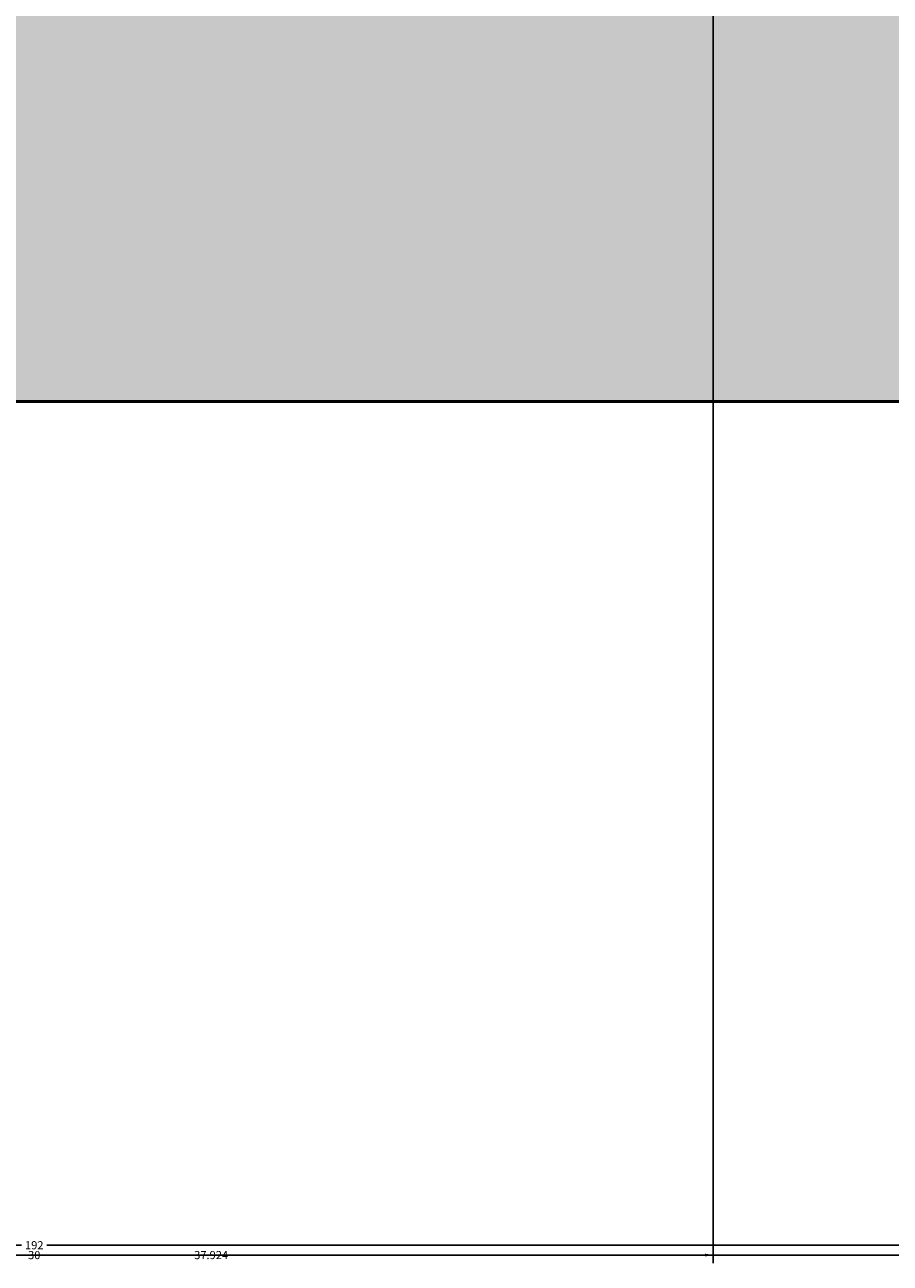
# Model space of a CAD drawing. Units: inches. Extents: x 2231 to 2461, y 2045 to 2455.
# Tile 14 of 95: x 2346 to 2365, y 2045 to 2072. Entities that reach past the tile are written whole.
import ezdxf

# ---------------------------------------------------------------- set-up
doc = ezdxf.new("R2010")
doc.units = ezdxf.units.IN
doc.layers.add('A-ANNO-DIMS', color=2, linetype='Continuous', lineweight=18)
doc.layers.add('A-WALL', color=7, linetype='Continuous', lineweight=50)
doc.layers.add('A-WALL-PATT', color=18, linetype='Continuous', lineweight=13, true_color=0x000000)
doc.styles.get("Standard").update_dxf_attribs({"font": 'arial.ttf'})
doc.dimstyles.get("Standard").update_dxf_attribs({"dimtxt": 0.18, "dimasz": 0.18, "dimexe": 0.18, "dimexo": 0.0625, "dimgap": 0.09, "dimtad": 0, "dimtih": 1, "dimtoh": 1, "dimdec": 4, "dimzin": 0, "dimdsep": 46, "dimtxsty": 'Standard', "dimcen": 0.09, "dimadec": 0, "dimazin": 0, "dimtfac": 1, "dimtdec": 4, "dimtofl": 0, "dimtmove": 0, "dimatfit": 3, "dimfxl": 1, "dimtolj": 1, "dimtzin": 0, "dimarcsym": 0})

# ---------------------------------------------------------------- blocks, each defined once
blk = doc.blocks.new('*D33')
at = {"layer": 'A-ANNO-DIMS', "color": 0, "lineweight": -2, "transparency": 16777216}
for p, q in [((2249.794, 2063.77), (2249.794, 2045.02)), ((2441.794, 2063.77), (2441.794, 2045.02)), ((2249.974, 2045.2), (2345.514, 2045.2)), ((2441.614, 2045.2), (2346.073, 2045.2))]:
    blk.add_line(p, q, dxfattribs=at)
at = {"layer": 'A-ANNO-DIMS', "color": 0, "transparency": 16777216}
for points in [[(2249.974, 2045.23), (2249.974, 2045.17), (2249.794, 2045.2)], [(2441.614, 2045.23), (2441.614, 2045.17), (2441.794, 2045.2)]]:
    blk.add_solid(points, dxfattribs=at)
at = {"layer": 'Defpoints', "color": 0, "transparency": 16777216}
for p in [(2249.794, 2063.833), (2441.794, 2063.833), (2249.794, 2045.2)]:
    blk.add_point(p, dxfattribs=at)
at = {"layer": 'A-ANNO-DIMS', "color": 0, "transparency": 16777216, "insert": (2345.794, 2045.2), "char_height": 0.18, "attachment_point": 5}
blk.add_mtext('\\A1;192', dxfattribs=at)
blk = doc.blocks.new('*D46')
at = {"layer": 'A-ANNO-DIMS', "color": 0, "lineweight": -2, "transparency": 16777216}
for p, q in [((2330.74, 2063.77), (2330.74, 2044.803)), ((2368.664, 2063.77), (2368.664, 2044.803)), ((2330.92, 2044.983), (2349.239, 2044.983)), ((2368.484, 2044.983), (2350.165, 2044.983))]:
    blk.add_line(p, q, dxfattribs=at)
at = {"layer": 'A-ANNO-DIMS', "color": 0, "transparency": 16777216}
for points in [[(2330.92, 2045.013), (2330.92, 2044.953), (2330.74, 2044.983)], [(2368.484, 2045.013), (2368.484, 2044.953), (2368.664, 2044.983)]]:
    blk.add_solid(points, dxfattribs=at)
at = {"layer": 'Defpoints', "color": 0, "transparency": 16777216}
for p in [(2330.74, 2063.833), (2368.664, 2063.833), (2368.664, 2044.983)]:
    blk.add_point(p, dxfattribs=at)
at = {"layer": 'A-ANNO-DIMS', "color": 0, "transparency": 16777216, "insert": (2349.702, 2044.983), "char_height": 0.18, "attachment_point": 5}
blk.add_mtext('\\A1;37.924', dxfattribs=at)
blk = doc.blocks.new('*D52')
at = {"layer": 'A-ANNO-DIMS', "color": 0, "lineweight": -2, "transparency": 16777216}
for p, q in [((2330.794, 2306.77), (2330.794, 2044.803)), ((2360.794, 2306.77), (2360.794, 2044.803)), ((2330.974, 2044.983), (2345.575, 2044.983)), ((2360.614, 2044.983), (2346.012, 2044.983))]:
    blk.add_line(p, q, dxfattribs=at)
at = {"layer": 'A-ANNO-DIMS', "color": 0, "transparency": 16777216}
for points in [[(2330.974, 2045.013), (2330.974, 2044.953), (2330.794, 2044.983)], [(2360.614, 2045.013), (2360.614, 2044.953), (2360.794, 2044.983)]]:
    blk.add_solid(points, dxfattribs=at)
at = {"layer": 'Defpoints', "color": 0, "transparency": 16777216}
for p in [(2330.794, 2306.833), (2360.794, 2306.833), (2360.794, 2044.983)]:
    blk.add_point(p, dxfattribs=at)
at = {"layer": 'A-ANNO-DIMS', "color": 0, "transparency": 16777216, "insert": (2345.794, 2044.983), "char_height": 0.18, "attachment_point": 5}
blk.add_mtext('\\A1;30', dxfattribs=at)
blk = doc.blocks.new('*D69')
at = {"layer": 'A-ANNO-DIMS', "color": 0, "lineweight": -2, "transparency": 16777216}
for p, q in [((2340.667, 2189.285), (2340.667, 2044.803)), ((2394.794, 2186.77), (2394.794, 2044.803)), ((2340.847, 2044.983), (2367.337, 2044.983)), ((2394.614, 2044.983), (2368.124, 2044.983))]:
    blk.add_line(p, q, dxfattribs=at)
at = {"layer": 'A-ANNO-DIMS', "color": 0, "transparency": 16777216}
for points in [[(2340.847, 2045.013), (2340.847, 2044.953), (2340.667, 2044.983)], [(2394.614, 2045.013), (2394.614, 2044.953), (2394.794, 2044.983)]]:
    blk.add_solid(points, dxfattribs=at)
at = {"layer": 'Defpoints', "color": 0, "transparency": 16777216}
for p in [(2340.667, 2189.348), (2394.794, 2186.833), (2394.794, 2044.983)]:
    blk.add_point(p, dxfattribs=at)
at = {"layer": 'A-ANNO-DIMS', "color": 0, "transparency": 16777216, "insert": (2367.73, 2044.983), "char_height": 0.18, "attachment_point": 5}
blk.add_mtext('\\A1;54.13', dxfattribs=at)

msp = doc.modelspace()

# ---------------------------------------------------------------- hatches: boundary and pattern name
at = {"layer": 'A-WALL-PATT'}
h = msp.add_hatch(color=256, dxfattribs=at)
h.dxf.hatch_style = 1
h.paths.add_polyline_path([(2441.7935, 2269.1535), (2432.7935, 2269.1535), (2432.7935, 2186.8328), (2396.7935, 2186.8328), (2396.7935, 2286.8328), (2394.7935, 2286.8328), (2394.7935, 2186.8328), (2334.7935, 2186.8328), (2334.7935, 2182.8328), (2432.7935, 2182.8328), (2432.7935, 2072.8328), (2416.6639, 2072.8328), (2416.6639, 2063.8328), (2441.7935, 2063.8328)])
h.paths.add_polyline_path([(2368.6639, 2072.8328), (2367.04, 2072.8328), (2330.7942, 2072.8328), (2330.7397, 2063.8328), (2368.6639, 2063.8328)])
h.paths.add_polyline_path([(2300.7392, 2068.3328), (2300.7392, 2072.8328), (2298.7935, 2072.8328), (2294.7935, 2072.8328), (2258.7935, 2072.8328), (2258.7935, 2120.8328), (2294.7935, 2120.8328), (2298.7935, 2120.8328), (2298.7935, 2128.8328), (2294.7935, 2128.8328), (2294.7935, 2124.8328), (2258.7935, 2124.8328), (2258.7935, 2182.8328), (2294.7935, 2182.8328), (2294.7935, 2174.8328), (2298.7935, 2174.8328), (2298.7935, 2182.8328), (2304.7935, 2182.8328), (2304.7935, 2186.8328), (2258.7935, 2186.8328), (2258.7935, 2221.999), (2249.7935, 2221.999), (2249.7935, 2063.8328), (2300.7392, 2063.8328)])
h.paths.add_polyline_path([(2391.9338, 2435.8328), (2333.82, 2435.8328), (2333.82, 2426.8328), (2368.7935, 2426.8328), (2368.7935, 2374.9508), (2368.7935, 2370.8328), (2372.3935, 2370.8328), (2372.7935, 2370.8328), (2372.7935, 2426.8328), (2391.9338, 2426.8328)])
h.paths.add_polyline_path([(2441.7935, 2435.8328), (2415.9338, 2435.8328), (2415.9338, 2426.8328), (2432.7935, 2426.8328), (2432.7935, 2334.8328), (2372.7935, 2334.8328), (2372.7935, 2346.8328), (2368.7935, 2346.8328), (2368.7935, 2306.8328), (2360.7935, 2306.8328), (2360.7935, 2302.8328), (2368.7935, 2302.8328), (2372.7935, 2302.8328), (2372.7935, 2330.8328), (2432.7935, 2330.8328), (2432.7935, 2317.1535), (2441.7935, 2317.1535)])
h.paths.add_polyline_path([(2285.82, 2435.8328), (2249.7935, 2435.8328), (2249.7935, 2269.999), (2258.7935, 2269.999), (2258.7935, 2302.8328), (2318.8168, 2302.8328), (2330.7935, 2302.8328), (2330.7935, 2306.8328), (2258.7935, 2306.8328), (2258.7935, 2426.8328), (2285.82, 2426.8328)])

# ---------------------------------------------------------------- linework, layer by layer
at = {"layer": 'A-WALL'}
msp.add_lwpolyline([(2300.7392, 2063.8328), (2249.7935, 2063.8328), (2249.7935, 2435.8328), (2441.7935, 2435.8328), (2441.7935, 2063.8328), (2330.7397, 2063.8328)], dxfattribs=at)

# ---------------------------------------------------------------- dimensions: what is measured, and where the dimension line sits
at = {"layer": 'A-ANNO-DIMS'}
for base, p1, p2, override, picture, middle in [((2360.7935, 2044.9825), (2330.7935, 2306.8328), (2360.7935, 2306.8328), {"dimdec": 0, "dimlfac": 1, "dimrnd": 0, "dimzin": 0, "dimdsep": 46, "dimlunit": 2}, '*D52', (2345.7935, 2044.9825)), ((2394.7935, 2044.9825), (2340.6673, 2189.3477), (2394.7935, 2186.8328), {"dimdec": 2, "dimlfac": 1, "dimrnd": 0, "dimzin": 0, "dimdsep": 46, "dimlunit": 2}, '*D69', (2367.7304, 2044.9825)), ((2368.6639, 2044.9825), (2330.7397, 2063.8328), (2368.6639, 2063.8328), {"dimdec": 3, "dimlfac": 1, "dimrnd": 0, "dimzin": 0, "dimdsep": 46, "dimlunit": 2}, '*D46', (2349.7018, 2044.9825))]:
    dim = msp.add_linear_dim(base=base, p1=p1, p2=p2, dimstyle='Standard', override=override, dxfattribs=at)
    dim.commit()
    dim.dimension.update_dxf_attribs({"geometry": picture, "text_midpoint": middle})
dim = msp.add_linear_dim(base=(2249.7935, 2045.2003), p1=(2441.7935, 2063.8328), p2=(2249.7935, 2063.8328), angle=180, dimstyle='Standard', override={"dimdec": 0, "dimlfac": 1, "dimrnd": 0, "dimzin": 0, "dimdsep": 46, "dimlunit": 2}, dxfattribs=at)
dim.commit()
dim.dimension.update_dxf_attribs({"geometry": '*D33', "text_midpoint": (2345.7935, 2045.2003)})

doc.saveas('drawing.dxf')
